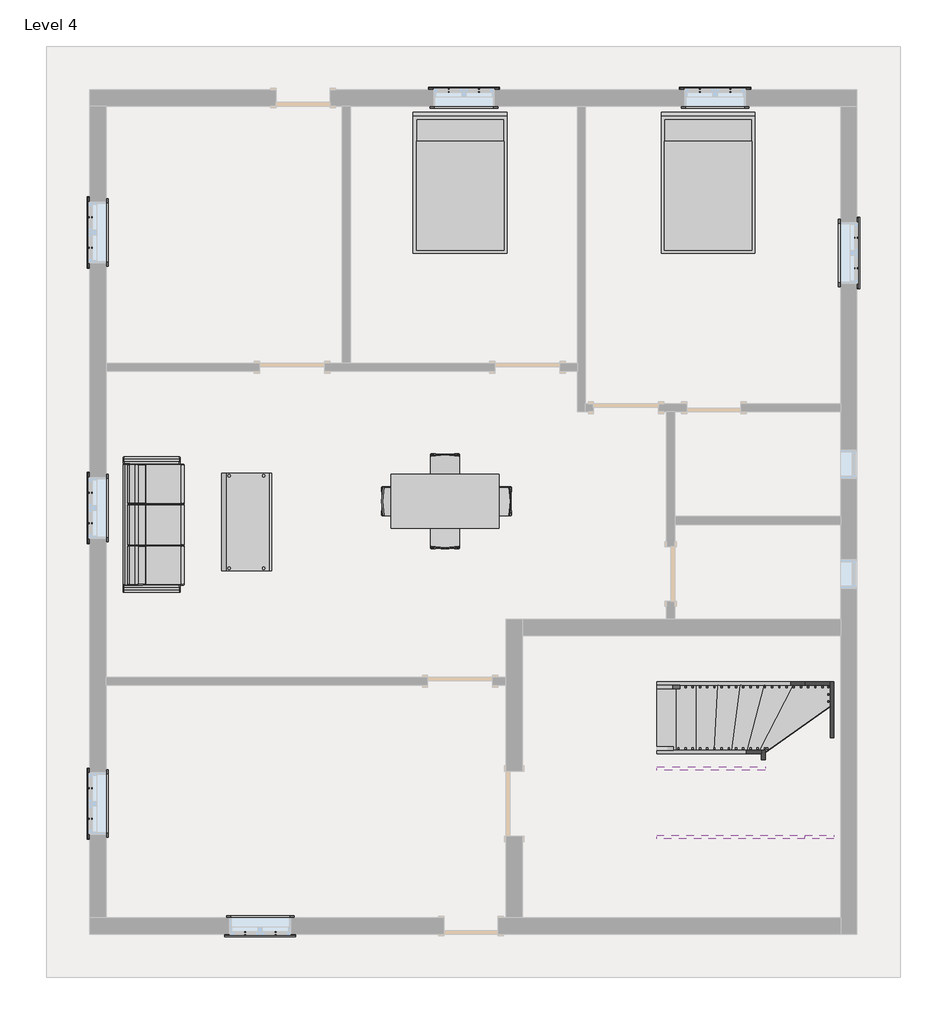
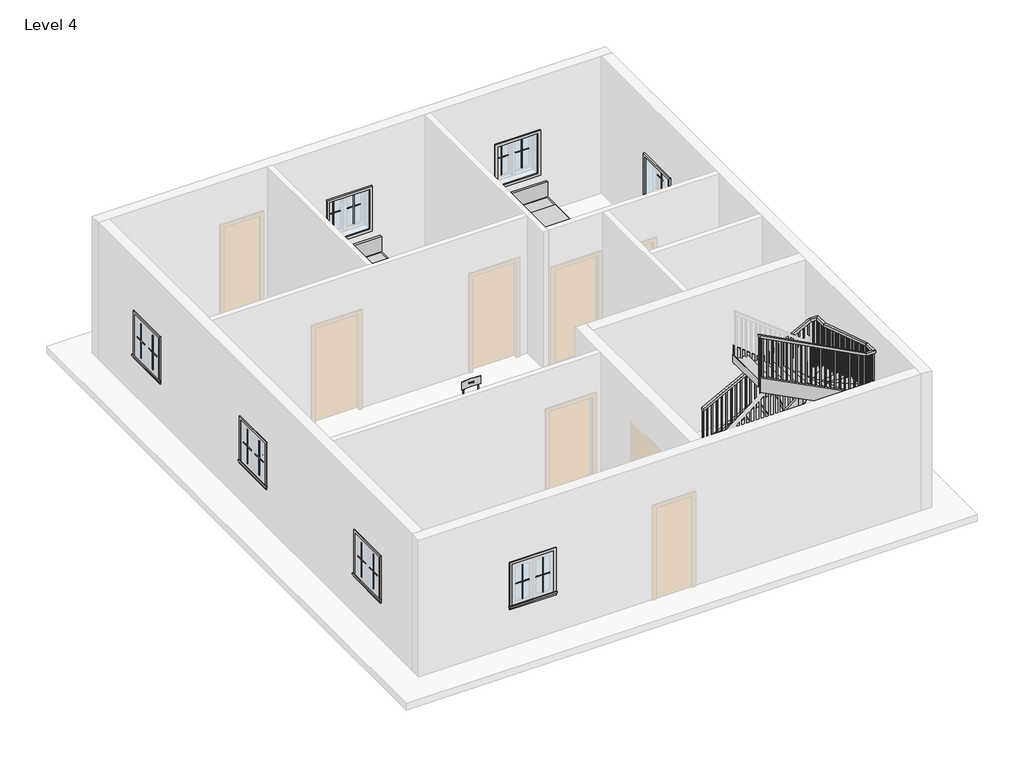
# One storey, part 2 of 2: 29 proxies, 8 members, 4 furniture elements, 1 railing, 1 stair flight.
"""IFC4 building model written with IfcOpenShell, lengths in millimetres."""

from ifc_helpers import new_model, si_unit, frame, origin, place, context, project, spatial, polyline, outline, extrude, faceted_brep, transform, mapped, element, save
from components import modern_coffee_table_17989_modern_coffee_table_17989_d3a860c8, muntin_pattern_2x2_muntin_pattern_2x2_b3fe6957, muntin_pattern_2x2_muntin_pattern_2x2_3e0ecaf2, trim_window_exterior_flat_with_sill_41619996, trim_window_interior_flat_picture_frame_51c85655, furniture_2fc85b74, furniture_29a9adb8, furniture_57072a26, bed_17739_bed_17739_15c61121, dining_table_w_chairs_11374_0cdfc61b, stair_flight_4d9189d9

model = new_model("IFC4")

# Units and contexts
model_context = context("Model", 3, world=origin())
ifc_project = project(units=[si_unit("LENGTHUNIT", "METRE", prefix="MILLI")], contexts=[model_context])

# Site, building, storey
site = spatial("IfcSite", under=ifc_project)
building = spatial("IfcBuilding", under=site)
storey = spatial("IfcBuildingStorey", under=building, Name="Level 4", Elevation=6400.8)

# Proxies
placement = place(None, origin())
modern_coffee_table_17989_modern_coffee_table_17989_shape = modern_coffee_table_17989_modern_coffee_table_17989_d3a860c8(model_context)
element("IfcBuildingElementProxy", 1, Name="Modern_Coffee_Table_17989 : Modern_Coffee_Table_17989", ObjectType="Modern_Coffee_Table_17989 : Modern_Coffee_Table_17989", at=placement, inside=storey, context=model_context, shape_type="MappedRepresentation", body=[
    mapped(modern_coffee_table_17989_modern_coffee_table_17989_shape, transform((-4791.7841049, 1283.3840961, 6400.8), x_axis=(0.0, 1.0, 0.0), y_axis=(-1.0, 0.0, 0.0), z_axis=(0.0, 0.0, 1.0))),
])
muntin_pattern_2x2_muntin_pattern_2x2_shape = muntin_pattern_2x2_muntin_pattern_2x2_b3fe6957(model_context)
element("IfcBuildingElementProxy", 2, Name="Muntin Pattern_2x2 : Muntin Pattern_2x2", ObjectType="Muntin Pattern_2x2 : Muntin Pattern_2x2", at=placement, inside=storey, context=model_context, shape_type="MappedRepresentation", body=[
    mapped(muntin_pattern_2x2_muntin_pattern_2x2_shape, transform((-1586.7442864, 7129.6784997, 7385.05), x_axis=(1.0, 0.0, 0.0), y_axis=(0.0, 1.0, 0.0), z_axis=(0.0, 0.0, 1.0))),
])
element("IfcBuildingElementProxy", 3, Name="Muntin Pattern_2x2 : Muntin Pattern_2x2", ObjectType="Muntin Pattern_2x2 : Muntin Pattern_2x2", at=placement, inside=storey, context=model_context, shape_type="MappedRepresentation", body=[
    mapped(muntin_pattern_2x2_muntin_pattern_2x2_shape, transform((1952.1107136, 7129.6784997, 7385.05), x_axis=(1.0, 0.0, 0.0), y_axis=(0.0, 1.0, 0.0), z_axis=(0.0, 0.0, 1.0))),
])
element("IfcBuildingElementProxy", 4, Name="Muntin Pattern_2x2 : Muntin Pattern_2x2", ObjectType="Muntin Pattern_2x2 : Muntin Pattern_2x2", at=placement, inside=storey, context=model_context, shape_type="MappedRepresentation", body=[
    mapped(muntin_pattern_2x2_muntin_pattern_2x2_shape, transform((-6633.4067864, 4915.1159997, 7385.05), x_axis=(0.0, 1.0, 0.0), y_axis=(-1.0, 0.0, 0.0), z_axis=(0.0, 0.0, 1.0))),
])
element("IfcBuildingElementProxy", 5, Name="Muntin Pattern_2x2 : Muntin Pattern_2x2", ObjectType="Muntin Pattern_2x2 : Muntin Pattern_2x2", at=placement, inside=storey, context=model_context, shape_type="MappedRepresentation", body=[
    mapped(muntin_pattern_2x2_muntin_pattern_2x2_shape, transform((-6633.4067864, 1038.4409997, 7385.05), x_axis=(0.0, 1.0, 0.0), y_axis=(-1.0, 0.0, 0.0), z_axis=(0.0, 0.0, 1.0))),
])
element("IfcBuildingElementProxy", 6, Name="Muntin Pattern_2x2 : Muntin Pattern_2x2", ObjectType="Muntin Pattern_2x2 : Muntin Pattern_2x2", at=placement, inside=storey, context=model_context, shape_type="MappedRepresentation", body=[
    mapped(muntin_pattern_2x2_muntin_pattern_2x2_shape, transform((4152.7032136, 5057.9909997, 7385.05), x_axis=(0.0, -1.0, 0.0), y_axis=(1.0, 0.0, 0.0), z_axis=(0.0, 0.0, 1.0))),
])
element("IfcBuildingElementProxy", 7, Name="Muntin Pattern_2x2 : Muntin Pattern_2x2", ObjectType="Muntin Pattern_2x2 : Muntin Pattern_2x2", at=placement, inside=storey, context=model_context, shape_type="MappedRepresentation", body=[
    mapped(muntin_pattern_2x2_muntin_pattern_2x2_shape, transform((-6633.4067864, -3125.2540003, 7385.05), x_axis=(0.0, 1.0, 0.0), y_axis=(-1.0, 0.0, 0.0), z_axis=(0.0, 0.0, 1.0))),
])
element("IfcBuildingElementProxy", 8, Name="Muntin Pattern_2x2 : Muntin Pattern_2x2", ObjectType="Muntin Pattern_2x2 : Muntin Pattern_2x2", at=placement, inside=storey, context=model_context, shape_type="MappedRepresentation", body=[
    mapped(muntin_pattern_2x2_muntin_pattern_2x2_shape, transform((-4028.3192864, -4738.4715003, 7385.05), x_axis=(-1.0, 0.0, 0.0), y_axis=(0.0, -1.0, 0.0), z_axis=(0.0, 0.0, 1.0))),
])
muntin_pattern_2x2_muntin_pattern_2x2_2_shape = muntin_pattern_2x2_muntin_pattern_2x2_3e0ecaf2(model_context)
element("IfcBuildingElementProxy", 9, Name="Muntin Pattern_2x2 : Muntin Pattern_2x2", ObjectType="Muntin Pattern_2x2 : Muntin Pattern_2x2", at=placement, inside=storey, context=model_context, shape_type="MappedRepresentation", body=[
    mapped(muntin_pattern_2x2_muntin_pattern_2x2_2_shape, transform((-1158.1192864, 7129.6784997, 7385.05), x_axis=(-1.0, 0.0, 0.0), y_axis=(0.0, -1.0, 0.0), z_axis=(0.0, 0.0, 1.0))),
])
element("IfcBuildingElementProxy", 10, Name="Muntin Pattern_2x2 : Muntin Pattern_2x2", ObjectType="Muntin Pattern_2x2 : Muntin Pattern_2x2", at=placement, inside=storey, context=model_context, shape_type="MappedRepresentation", body=[
    mapped(muntin_pattern_2x2_muntin_pattern_2x2_2_shape, transform((2380.7357136, 7129.6784997, 7385.05), x_axis=(-1.0, 0.0, 0.0), y_axis=(0.0, -1.0, 0.0), z_axis=(0.0, 0.0, 1.0))),
])
element("IfcBuildingElementProxy", 11, Name="Muntin Pattern_2x2 : Muntin Pattern_2x2", ObjectType="Muntin Pattern_2x2 : Muntin Pattern_2x2", at=placement, inside=storey, context=model_context, shape_type="MappedRepresentation", body=[
    mapped(muntin_pattern_2x2_muntin_pattern_2x2_2_shape, transform((-6633.4067864, 5343.7409997, 7385.05), x_axis=(0.0, -1.0, 0.0), y_axis=(1.0, 0.0, 0.0), z_axis=(0.0, 0.0, 1.0))),
])
element("IfcBuildingElementProxy", 12, Name="Muntin Pattern_2x2 : Muntin Pattern_2x2", ObjectType="Muntin Pattern_2x2 : Muntin Pattern_2x2", at=placement, inside=storey, context=model_context, shape_type="MappedRepresentation", body=[
    mapped(muntin_pattern_2x2_muntin_pattern_2x2_2_shape, transform((-6633.4067864, 1467.0659997, 7385.05), x_axis=(0.0, -1.0, 0.0), y_axis=(1.0, 0.0, 0.0), z_axis=(0.0, 0.0, 1.0))),
])
element("IfcBuildingElementProxy", 13, Name="Muntin Pattern_2x2 : Muntin Pattern_2x2", ObjectType="Muntin Pattern_2x2 : Muntin Pattern_2x2", at=placement, inside=storey, context=model_context, shape_type="MappedRepresentation", body=[
    mapped(muntin_pattern_2x2_muntin_pattern_2x2_2_shape, transform((4152.7032136, 4629.3659997, 7385.05), x_axis=(0.0, 1.0, 0.0), y_axis=(-1.0, 0.0, 0.0), z_axis=(0.0, 0.0, 1.0))),
])
element("IfcBuildingElementProxy", 14, Name="Muntin Pattern_2x2 : Muntin Pattern_2x2", ObjectType="Muntin Pattern_2x2 : Muntin Pattern_2x2", at=placement, inside=storey, context=model_context, shape_type="MappedRepresentation", body=[
    mapped(muntin_pattern_2x2_muntin_pattern_2x2_2_shape, transform((-6633.4067864, -2696.6290003, 7385.05), x_axis=(0.0, -1.0, 0.0), y_axis=(1.0, 0.0, 0.0), z_axis=(0.0, 0.0, 1.0))),
])
element("IfcBuildingElementProxy", 15, Name="Muntin Pattern_2x2 : Muntin Pattern_2x2", ObjectType="Muntin Pattern_2x2 : Muntin Pattern_2x2", at=placement, inside=storey, context=model_context, shape_type="MappedRepresentation", body=[
    mapped(muntin_pattern_2x2_muntin_pattern_2x2_2_shape, transform((-4456.9442864, -4738.4715003, 7385.05), x_axis=(1.0, 0.0, 0.0), y_axis=(0.0, 1.0, 0.0), z_axis=(0.0, 0.0, 1.0))),
])
trim_window_exterior_flat_with_sill_shape = trim_window_exterior_flat_with_sill_41619996(model_context)
element("IfcBuildingElementProxy", 16, Name="Trim-Window-Exterior-Flat : with Sill", ObjectType="Trim-Window-Exterior-Flat : with Sill", at=placement, inside=storey, context=model_context, shape_type="MappedRepresentation", body=[
    mapped(trim_window_exterior_flat_with_sill_shape, transform((-1372.4317864, 7139.2034997, 8229.6), x_axis=(-1.0, 0.0, 0.0), y_axis=(0.0, 0.0, 1.0), z_axis=(0.0, 1.0, 0.0))),
])
element("IfcBuildingElementProxy", 17, Name="Trim-Window-Exterior-Flat : with Sill", ObjectType="Trim-Window-Exterior-Flat : with Sill", at=placement, inside=storey, context=model_context, shape_type="MappedRepresentation", body=[
    mapped(trim_window_exterior_flat_with_sill_shape, transform((2166.4232136, 7139.2034997, 8229.6), x_axis=(-1.0, 0.0, 0.0), y_axis=(0.0, 0.0, 1.0), z_axis=(0.0, 1.0, 0.0))),
])
element("IfcBuildingElementProxy", 18, Name="Trim-Window-Exterior-Flat : with Sill", ObjectType="Trim-Window-Exterior-Flat : with Sill", at=placement, inside=storey, context=model_context, shape_type="MappedRepresentation", body=[
    mapped(trim_window_exterior_flat_with_sill_shape, transform((-6642.9317864, 5129.4284997, 8229.6), x_axis=(0.0, -1.0, 0.0), y_axis=(0.0, 0.0, 1.0), z_axis=(-1.0, 0.0, 0.0))),
])
element("IfcBuildingElementProxy", 19, Name="Trim-Window-Exterior-Flat : with Sill", ObjectType="Trim-Window-Exterior-Flat : with Sill", at=placement, inside=storey, context=model_context, shape_type="MappedRepresentation", body=[
    mapped(trim_window_exterior_flat_with_sill_shape, transform((-6642.9317864, 1252.7534997, 8229.6), x_axis=(0.0, -1.0, 0.0), y_axis=(0.0, 0.0, 1.0), z_axis=(-1.0, 0.0, 0.0))),
])
element("IfcBuildingElementProxy", 20, Name="Trim-Window-Exterior-Flat : with Sill", ObjectType="Trim-Window-Exterior-Flat : with Sill", at=placement, inside=storey, context=model_context, shape_type="MappedRepresentation", body=[
    mapped(trim_window_exterior_flat_with_sill_shape, transform((4162.2282136, 4843.6784997, 8229.6), x_axis=(0.0, 1.0, 0.0), y_axis=(0.0, 0.0, 1.0), z_axis=(1.0, 0.0, 0.0))),
])
element("IfcBuildingElementProxy", 21, Name="Trim-Window-Exterior-Flat : with Sill", ObjectType="Trim-Window-Exterior-Flat : with Sill", at=placement, inside=storey, context=model_context, shape_type="MappedRepresentation", body=[
    mapped(trim_window_exterior_flat_with_sill_shape, transform((-6642.9317864, -2910.9415003, 8229.6), x_axis=(0.0, -1.0, 0.0), y_axis=(0.0, 0.0, 1.0), z_axis=(-1.0, 0.0, 0.0))),
])
element("IfcBuildingElementProxy", 22, Name="Trim-Window-Exterior-Flat : with Sill", ObjectType="Trim-Window-Exterior-Flat : with Sill", at=placement, inside=storey, context=model_context, shape_type="MappedRepresentation", body=[
    mapped(trim_window_exterior_flat_with_sill_shape, transform((-4242.6317864, -4747.9965003, 8229.6), x_axis=(1.0, 0.0, 0.0), y_axis=(0.0, 0.0, 1.0), z_axis=(0.0, -1.0, 0.0))),
])
trim_window_interior_flat_picture_frame_shape = trim_window_interior_flat_picture_frame_51c85655(model_context)
element("IfcBuildingElementProxy", 23, Name="Trim-Window-Interior-Flat : Picture Frame", ObjectType="Trim-Window-Interior-Flat : Picture Frame", at=placement, inside=storey, context=model_context, shape_type="MappedRepresentation", body=[
    mapped(trim_window_interior_flat_picture_frame_shape, transform((-1372.4317864, 6910.6034997, 8229.6), x_axis=(1.0, 0.0, 0.0), y_axis=(0.0, 0.0, 1.0), z_axis=(0.0, -1.0, 0.0))),
])
element("IfcBuildingElementProxy", 24, Name="Trim-Window-Interior-Flat : Picture Frame", ObjectType="Trim-Window-Interior-Flat : Picture Frame", at=placement, inside=storey, context=model_context, shape_type="MappedRepresentation", body=[
    mapped(trim_window_interior_flat_picture_frame_shape, transform((2166.4232136, 6910.6034997, 8229.6), x_axis=(1.0, 0.0, 0.0), y_axis=(0.0, 0.0, 1.0), z_axis=(0.0, -1.0, 0.0))),
])
element("IfcBuildingElementProxy", 25, Name="Trim-Window-Interior-Flat : Picture Frame", ObjectType="Trim-Window-Interior-Flat : Picture Frame", at=placement, inside=storey, context=model_context, shape_type="MappedRepresentation", body=[
    mapped(trim_window_interior_flat_picture_frame_shape, transform((-6414.3317864, 5129.4284997, 8229.6), x_axis=(0.0, 1.0, 0.0), y_axis=(0.0, 0.0, 1.0), z_axis=(1.0, 0.0, 0.0))),
])
element("IfcBuildingElementProxy", 26, Name="Trim-Window-Interior-Flat : Picture Frame", ObjectType="Trim-Window-Interior-Flat : Picture Frame", at=placement, inside=storey, context=model_context, shape_type="MappedRepresentation", body=[
    mapped(trim_window_interior_flat_picture_frame_shape, transform((-6414.3317864, 1252.7534997, 8229.6), x_axis=(0.0, 1.0, 0.0), y_axis=(0.0, 0.0, 1.0), z_axis=(1.0, 0.0, 0.0))),
])
element("IfcBuildingElementProxy", 27, Name="Trim-Window-Interior-Flat : Picture Frame", ObjectType="Trim-Window-Interior-Flat : Picture Frame", at=placement, inside=storey, context=model_context, shape_type="MappedRepresentation", body=[
    mapped(trim_window_interior_flat_picture_frame_shape, transform((3933.6282136, 4843.6784997, 8229.6), x_axis=(0.0, -1.0, 0.0), y_axis=(0.0, 0.0, 1.0), z_axis=(-1.0, 0.0, 0.0))),
])
element("IfcBuildingElementProxy", 28, Name="Trim-Window-Interior-Flat : Picture Frame", ObjectType="Trim-Window-Interior-Flat : Picture Frame", at=placement, inside=storey, context=model_context, shape_type="MappedRepresentation", body=[
    mapped(trim_window_interior_flat_picture_frame_shape, transform((-6414.3317864, -2910.9415003, 8229.6), x_axis=(0.0, 1.0, 0.0), y_axis=(0.0, 0.0, 1.0), z_axis=(1.0, 0.0, 0.0))),
])
element("IfcBuildingElementProxy", 29, Name="Trim-Window-Interior-Flat : Picture Frame", ObjectType="Trim-Window-Interior-Flat : Picture Frame", at=placement, inside=storey, context=model_context, shape_type="MappedRepresentation", body=[
    mapped(trim_window_interior_flat_picture_frame_shape, transform((-4242.6317864, -4519.3965003, 8229.6), x_axis=(-1.0, 0.0, 0.0), y_axis=(0.0, 0.0, 1.0), z_axis=(0.0, 1.0, 0.0))),
])

# Furniture
furniture_shape = furniture_2fc85b74(model_context)
furniture_2_shape = furniture_29a9adb8(model_context)
furniture_3_shape = furniture_57072a26(model_context)
element("IfcFurniture", 30, at=placement, inside=storey, context=model_context, shape_type="MappedRepresentation", body=[
    mapped(furniture_shape, transform((-5371.0104604, 1017.8034997, 6400.8), x_axis=(0.0, 1.0, 0.0), y_axis=(-1.0, 0.0, 0.0), z_axis=(0.0, 0.0, 1.0))),
    mapped(furniture_2_shape, transform((-5371.0104604, 1017.8034997, 6400.8), x_axis=(0.0, 1.0, 0.0), y_axis=(-1.0, 0.0, 0.0), z_axis=(0.0, 0.0, 1.0))),
    mapped(furniture_3_shape, transform((-5371.0104604, 1017.8034997, 6400.8), x_axis=(0.0, 1.0, 0.0), y_axis=(-1.0, 0.0, 0.0), z_axis=(0.0, 0.0, 1.0))),
])
bed_17739_bed_17739_shape = bed_17739_bed_17739_15c61121(model_context)
element("IfcFurniture", 31, ObjectType="Bed_17739 : Bed_17739", at=placement, inside=storey, context=model_context, shape_type="MappedRepresentation", body=[
    mapped(bed_17739_bed_17739_shape, transform((-1425.7717864, 5805.7034997, 6400.8), x_axis=(1.0, 0.0, 0.0), y_axis=(0.0, 1.0, 0.0), z_axis=(0.0, 0.0, 1.0))),
])
element("IfcFurniture", 32, ObjectType="Bed_17739 : Bed_17739", at=placement, inside=storey, context=model_context, shape_type="MappedRepresentation", body=[
    mapped(bed_17739_bed_17739_shape, transform((2066.7282136, 5805.7034997, 6400.8), x_axis=(1.0, 0.0, 0.0), y_axis=(0.0, 1.0, 0.0), z_axis=(0.0, 0.0, 1.0))),
])
dining_table_w_chairs_11374_shape = dining_table_w_chairs_11374_0cdfc61b(model_context)
element("IfcFurniture", 33, ObjectType="Dining_Table_w_Chairs_11374", at=placement, inside=storey, context=model_context, shape_type="MappedRepresentation", body=[
    mapped(dining_table_w_chairs_11374_shape, transform((-1657.0397106, 1252.0888157, 6400.8), x_axis=(1.0, 0.0, 0.0), y_axis=(0.0, 1.0, 0.0), z_axis=(0.0, 0.0, 1.0))),
])

# Members
element("IfcMember", 34, ObjectType="Stringer - 2\" Width", at=placement, inside=storey, context=model_context, shape_type="SweptSolid", body=[
    extrude(outline(polyline([(6630.439954, 1342.8282136), (6400.8, 1342.8282136), (6400.8, 1562.5905312), (7363.300629, 3430.2454053), (7706.1956453, 3430.2454053), (6630.439954, 1342.8282136)])), frame((0.0, -1245.3365003, 0.0), z_axis=(0.0, 1.0, 0.0), x_axis=(0.0, 0.0, 1.0)), (0.0, 0.0, 1.0), 50.8),
])
element("IfcMember", 35, ObjectType="Stringer - 2\" Width", at=placement, inside=storey, context=model_context, shape_type="SweptSolid", body=[
    extrude(outline(polyline([(3430.2454053, -1245.3365003), (3430.2454053, -1194.5365003), (3784.9599055, -1194.5365003), (3784.9599055, -1245.3365003), (3430.2454053, -1245.3365003)])), frame((0.0, 0.0, 7363.300629), z_axis=(0.0, 0.0, 1.0), x_axis=(1.0, 0.0, 0.0)), (0.0, 0.0, 1.0), 342.8950162),
])
element("IfcMember", 36, ObjectType="Stringer - 2\" Width", at=placement, inside=storey, context=model_context, shape_type="SweptSolid", body=[
    extrude(outline(polyline([(-1194.5365003, 7689.8952212), (-1194.5365003, 7401.3956453), (-1364.0589833, 7401.3956453), (-3353.5365003, 8039.7682298), (-3353.5365003, 8370.7972697), (-3316.5563831, 8370.7972697), (-1194.5365003, 7689.8952212)])), frame((3784.9599055, 0.0, 0.0), z_axis=(1.0, 0.0, 0.0), x_axis=(0.0, 1.0, 0.0)), (0.0, 0.0, 1.0), 50.8),
])
element("IfcMember", 37, ObjectType="Stringer - 2\" Width", at=placement, inside=storey, context=model_context, shape_type="SweptSolid", body=[
    extrude(outline(polyline([(3835.7599055, -3353.5365003), (3835.7599055, -3404.3365003), (3430.2454053, -3404.3365003), (3430.2454053, -3353.5365003), (3835.7599055, -3353.5365003)])), frame((0.0, 0.0, 8050.6904473), z_axis=(0.0, 0.0, 1.0), x_axis=(1.0, 0.0, 0.0)), (0.0, 0.0, 1.0), 320.1068224),
])
element("IfcMember", 38, ObjectType="Stringer - 2\" Width", at=placement, inside=storey, context=model_context, shape_type="SweptSolid", body=[
    extrude(outline(polyline([(8050.6904473, 3430.2454053), (8370.7972697, 3430.2454053), (9446.5529609, 1342.8282136), (9126.4461385, 1342.8282136), (8050.6904473, 3430.2454053)])), frame((0.0, -3404.3365003, 0.0), z_axis=(0.0, 1.0, 0.0), x_axis=(0.0, 0.0, 1.0)), (0.0, 0.0, 1.0), 50.8),
])
element("IfcMember", 39, ObjectType="Stringer - 2\" Width", at=placement, inside=storey, context=model_context, shape_type="SweptSolid", body=[
    extrude(outline(polyline([(6576.9764461, 1342.8282136), (6400.8, 1342.8282136), (6400.8, 1609.0898582), (7387.9410923, 2819.7599055), (7781.218648, 2819.7599055), (6576.9764461, 1342.8282136)])), frame((0.0, -2210.5365003, 0.0), z_axis=(0.0, 1.0, 0.0), x_axis=(0.0, 0.0, 1.0)), (0.0, 0.0, 1.0), 50.8),
])
element("IfcMember", 40, ObjectType="Stringer - 2\" Width", at=placement, inside=storey, context=model_context, shape_type="SweptSolid", body=[
    extrude(outline(polyline([(-2159.7365003, 7974.0682978), (-2159.7365003, 7429.3617647), (-2193.9787177, 7429.3617647), (-2388.3365003, 7761.265107), (-2388.3365003, 8326.9409689), (-2366.3736178, 8326.9409689), (-2159.7365003, 7974.0682978)])), frame((2819.7599055, 0.0, 0.0), z_axis=(1.0, 0.0, 0.0), x_axis=(0.0, 1.0, 0.0)), (0.0, 0.0, 1.0), 50.8),
])
element("IfcMember", 41, ObjectType="Stringer - 2\" Width", at=placement, inside=storey, context=model_context, shape_type="SweptSolid", body=[
    extrude(outline(polyline([(7933.6634131, 2870.5599055), (8326.9409689, 2870.5599055), (9572.6038432, 1342.8282136), (9179.3262875, 1342.8282136), (7933.6634131, 2870.5599055)])), frame((0.0, -2439.1365003, 0.0), z_axis=(0.0, 1.0, 0.0), x_axis=(0.0, 0.0, 1.0)), (0.0, 0.0, 1.0), 50.8),
])

# Railing
element("IfcRailing", 42, ObjectType="Handrail - Rectangular", at=placement, inside=storey, context=model_context, shape_type="SolidModel", body=[
    faceted_brep([(1342.8282136, -1245.3365003, 7484.5333333), (1342.8282136, -1245.3365003, 7427.0742652), (1342.8282136, -1296.1365003, 7427.0742652), (1342.8282136, -1296.1365003, 7484.5333333), (3600.5532757, -1245.3365003, 8677.8239201), (3613.1523402, -1245.3365003, 8627.0239201), (3613.1523402, -1296.1365003, 8627.0239201), (3600.5532757, -1296.1365003, 8677.8239201), (3784.9599055, -1245.3365003, 8677.8239201), (3784.9599055, -1245.3365003, 8627.0239201), (3734.1599055, -1296.1365003, 8627.0239201), (3734.1599055, -1296.1365003, 8677.8239201), (3784.9599055, -1532.6483825, 8677.8239201), (3784.9599055, -1540.5989586, 8627.0239201), (3734.1599055, -1540.5989586, 8627.0239201), (3734.1599055, -1532.6483825, 8677.8239201), (3784.9599055, -3066.2246182, 9169.9094132), (3784.9599055, -3074.1751943, 9119.1094132), (3734.1599055, -3074.1751943, 9119.1094132), (3734.1599055, -3066.2246182, 9169.9094132), (3784.9599055, -3353.5365003, 9169.9094132), (3784.9599055, -3353.5365003, 9119.1094132), (3734.1599055, -3302.7365003, 9119.1094132), (3734.1599055, -3302.7365003, 9169.9094132), (3600.5532757, -3353.5365003, 9169.9094132), (3587.9542112, -3353.5365003, 9119.1094132), (3587.9542112, -3302.7365003, 9119.1094132), (3600.5532757, -3302.7365003, 9169.9094132), (1342.8282136, -3353.5365003, 10363.2), (1342.8282136, -3302.7365003, 10363.2), (1342.8282136, -3302.7365003, 10305.7409318), (1342.8282136, -3353.5365003, 10305.7409318)], [[[0, 1, 2, 3]], [[1, 0, 4, 5]], [[2, 1, 5, 6]], [[3, 2, 6, 7]], [[0, 3, 7, 4]], [[5, 4, 8, 9]], [[6, 5, 9, 10]], [[7, 6, 10, 11]], [[4, 7, 11, 8]], [[9, 8, 12, 13]], [[10, 9, 13, 14]], [[11, 10, 14, 15]], [[8, 11, 15, 12]], [[13, 12, 16, 17]], [[14, 13, 17, 18]], [[15, 14, 18, 19]], [[12, 15, 19, 16]], [[17, 16, 20, 21]], [[18, 17, 21, 22]], [[19, 18, 22, 23]], [[16, 19, 23, 20]], [[21, 20, 24, 25]], [[22, 21, 25, 26]], [[23, 22, 26, 27]], [[20, 23, 27, 24]], [[28, 29, 30, 31]], [[25, 24, 28, 31]], [[26, 25, 31, 30]], [[27, 26, 30, 29]], [[24, 27, 29, 28]]]),
    extrude(outline(polyline([(10268.5284102, 1413.2349055), (9279.4666667, 1413.2349055), (9279.4666667, 1432.2849055), (10258.4597858, 1432.2849055), (10268.5284102, 1413.2349055)])), frame((0.0, -3337.6615003, 0.0), z_axis=(0.0, 1.0, 0.0), x_axis=(0.0, 0.0, 1.0)), (0.0, 0.0, 1.0), 19.05),
    extrude(outline(polyline([(10214.82908, 1514.8349055), (9279.4666667, 1514.8349055), (9279.4666667, 1533.8849055), (10204.7604556, 1533.8849055), (10214.82908, 1514.8349055)])), frame((0.0, -3337.6615003, 0.0), z_axis=(0.0, 1.0, 0.0), x_axis=(0.0, 0.0, 1.0)), (0.0, 0.0, 1.0), 19.05),
    extrude(outline(polyline([(10161.1297498, 1616.4349055), (9110.1333333, 1616.4349055), (9110.1333333, 1635.4849055), (10151.0611254, 1635.4849055), (10161.1297498, 1616.4349055)])), frame((0.0, -3337.6615003, 0.0), z_axis=(0.0, 1.0, 0.0), x_axis=(0.0, 0.0, 1.0)), (0.0, 0.0, 1.0), 19.05),
    extrude(outline(polyline([(10107.4304196, 1718.0349055), (9110.1333333, 1718.0349055), (9110.1333333, 1737.0849055), (10097.3617952, 1737.0849055), (10107.4304196, 1718.0349055)])), frame((0.0, -3337.6615003, 0.0), z_axis=(0.0, 1.0, 0.0), x_axis=(0.0, 0.0, 1.0)), (0.0, 0.0, 1.0), 19.05),
    extrude(outline(polyline([(10053.7310894, 1819.6349055), (9110.1333333, 1819.6349055), (9110.1333333, 1838.6849055), (10043.662465, 1838.6849055), (10053.7310894, 1819.6349055)])), frame((0.0, -3337.6615003, 0.0), z_axis=(0.0, 1.0, 0.0), x_axis=(0.0, 0.0, 1.0)), (0.0, 0.0, 1.0), 19.05),
    extrude(outline(polyline([(10000.0317592, 1921.2349055), (8940.8, 1921.2349055), (8940.8, 1940.2849055), (9989.9631348, 1940.2849055), (10000.0317592, 1921.2349055)])), frame((0.0, -3337.6615003, 0.0), z_axis=(0.0, 1.0, 0.0), x_axis=(0.0, 0.0, 1.0)), (0.0, 0.0, 1.0), 19.05),
    extrude(outline(polyline([(9946.332429, 2022.8349055), (8940.8, 2022.8349055), (8940.8, 2041.8849055), (9936.2638046, 2041.8849055), (9946.332429, 2022.8349055)])), frame((0.0, -3337.6615003, 0.0), z_axis=(0.0, 1.0, 0.0), x_axis=(0.0, 0.0, 1.0)), (0.0, 0.0, 1.0), 19.05),
    extrude(outline(polyline([(9892.6330988, 2124.4349055), (8940.8, 2124.4349055), (8940.8, 2143.4849055), (9882.5644744, 2143.4849055), (9892.6330988, 2124.4349055)])), frame((0.0, -3337.6615003, 0.0), z_axis=(0.0, 1.0, 0.0), x_axis=(0.0, 0.0, 1.0)), (0.0, 0.0, 1.0), 19.05),
    extrude(outline(polyline([(9838.9337686, 2226.0349055), (8771.4666667, 2226.0349055), (8771.4666667, 2245.0849055), (9828.8651442, 2245.0849055), (9838.9337686, 2226.0349055)])), frame((0.0, -3337.6615003, 0.0), z_axis=(0.0, 1.0, 0.0), x_axis=(0.0, 0.0, 1.0)), (0.0, 0.0, 1.0), 19.05),
    extrude(outline(polyline([(9785.2344384, 2327.6349055), (8771.4666667, 2327.6349055), (8771.4666667, 2346.6849055), (9775.165814, 2346.6849055), (9785.2344384, 2327.6349055)])), frame((0.0, -3337.6615003, 0.0), z_axis=(0.0, 1.0, 0.0), x_axis=(0.0, 0.0, 1.0)), (0.0, 0.0, 1.0), 19.05),
    extrude(outline(polyline([(9731.5351082, 2429.2349055), (8771.4666667, 2429.2349055), (8771.4666667, 2448.2849055), (9721.4664838, 2448.2849055), (9731.5351082, 2429.2349055)])), frame((0.0, -3337.6615003, 0.0), z_axis=(0.0, 1.0, 0.0), x_axis=(0.0, 0.0, 1.0)), (0.0, 0.0, 1.0), 19.05),
    extrude(outline(polyline([(9677.835778, 2530.8349055), (8602.1333333, 2530.8349055), (8602.1333333, 2549.8849055), (9667.7671536, 2549.8849055), (9677.835778, 2530.8349055)])), frame((0.0, -3337.6615003, 0.0), z_axis=(0.0, 1.0, 0.0), x_axis=(0.0, 0.0, 1.0)), (0.0, 0.0, 1.0), 19.05),
    extrude(outline(polyline([(9624.1364478, 2632.4349055), (8602.1333333, 2632.4349055), (8602.1333333, 2651.4849055), (9614.0678234, 2651.4849055), (9624.1364478, 2632.4349055)])), frame((0.0, -3337.6615003, 0.0), z_axis=(0.0, 1.0, 0.0), x_axis=(0.0, 0.0, 1.0)), (0.0, 0.0, 1.0), 19.05),
    extrude(outline(polyline([(9570.4371176, 2734.0349055), (8602.1333333, 2734.0349055), (8602.1333333, 2753.0849055), (9560.3684932, 2753.0849055), (9570.4371176, 2734.0349055)])), frame((0.0, -3337.6615003, 0.0), z_axis=(0.0, 1.0, 0.0), x_axis=(0.0, 0.0, 1.0)), (0.0, 0.0, 1.0), 19.05),
    extrude(outline(polyline([(9516.7377874, 2835.6349055), (8602.1333333, 2835.6349055), (8602.1333333, 2854.6849055), (9506.669163, 2854.6849055), (9516.7377874, 2835.6349055)])), frame((0.0, -3337.6615003, 0.0), z_axis=(0.0, 1.0, 0.0), x_axis=(0.0, 0.0, 1.0)), (0.0, 0.0, 1.0), 19.05),
    extrude(outline(polyline([(9463.0384572, 2937.2349055), (8432.8, 2937.2349055), (8432.8, 2956.2849055), (9452.9698328, 2956.2849055), (9463.0384572, 2937.2349055)])), frame((0.0, -3337.6615003, 0.0), z_axis=(0.0, 1.0, 0.0), x_axis=(0.0, 0.0, 1.0)), (0.0, 0.0, 1.0), 19.05),
    extrude(outline(polyline([(9409.339127, 3038.8349055), (8432.8, 3038.8349055), (8432.8, 3057.8849055), (9399.2705026, 3057.8849055), (9409.339127, 3038.8349055)])), frame((0.0, -3337.6615003, 0.0), z_axis=(0.0, 1.0, 0.0), x_axis=(0.0, 0.0, 1.0)), (0.0, 0.0, 1.0), 19.05),
    extrude(outline(polyline([(9355.6397968, 3140.4349055), (8432.8, 3140.4349055), (8432.8, 3159.4849055), (9345.5711724, 3159.4849055), (9355.6397968, 3140.4349055)])), frame((0.0, -3337.6615003, 0.0), z_axis=(0.0, 1.0, 0.0), x_axis=(0.0, 0.0, 1.0)), (0.0, 0.0, 1.0), 19.05),
    extrude(outline(polyline([(9301.9404666, 3242.0349055), (8432.8, 3242.0349055), (8432.8, 3261.0849055), (9291.8718422, 3261.0849055), (9301.9404666, 3242.0349055)])), frame((0.0, -3337.6615003, 0.0), z_axis=(0.0, 1.0, 0.0), x_axis=(0.0, 0.0, 1.0)), (0.0, 0.0, 1.0), 19.05),
    extrude(outline(polyline([(9248.2411364, 3343.6349055), (8263.4666667, 3343.6349055), (8263.4666667, 3362.6849055), (9238.172512, 3362.6849055), (9248.2411364, 3343.6349055)])), frame((0.0, -3337.6615003, 0.0), z_axis=(0.0, 1.0, 0.0), x_axis=(0.0, 0.0, 1.0)), (0.0, 0.0, 1.0), 19.05),
    extrude(outline(polyline([(9194.5418062, 3445.2349055), (8263.4666667, 3445.2349055), (8263.4666667, 3464.2849055), (9184.4731818, 3464.2849055), (9194.5418062, 3445.2349055)])), frame((0.0, -3337.6615003, 0.0), z_axis=(0.0, 1.0, 0.0), x_axis=(0.0, 0.0, 1.0)), (0.0, 0.0, 1.0), 19.05),
    extrude(outline(polyline([(9140.842476, 3546.8349055), (8263.4666667, 3546.8349055), (8263.4666667, 3565.8849055), (9130.7738516, 3565.8849055), (9140.842476, 3546.8349055)])), frame((0.0, -3337.6615003, 0.0), z_axis=(0.0, 1.0, 0.0), x_axis=(0.0, 0.0, 1.0)), (0.0, 0.0, 1.0), 19.05),
    extrude(outline(polyline([(3667.4849055, -3337.6615003), (3648.4349055, -3337.6615003), (3648.4349055, -3318.6115003), (3667.4849055, -3318.6115003), (3667.4849055, -3337.6615003)])), frame((0.0, 0.0, 8263.4666667), z_axis=(0.0, 0.0, 1.0), x_axis=(1.0, 0.0, 0.0)), (0.0, 0.0, 1.0), 855.6427466),
    extrude(outline(polyline([(3769.0849055, -3293.2115003), (3769.0849055, -3312.2615003), (3750.0349055, -3312.2615003), (3750.0349055, -3293.2115003), (3769.0849055, -3293.2115003)])), frame((0.0, 0.0, 8263.4666667), z_axis=(0.0, 0.0, 1.0), x_axis=(1.0, 0.0, 0.0)), (0.0, 0.0, 1.0), 855.6427466),
    extrude(outline(polyline([(3769.0849055, -3191.6115003), (3769.0849055, -3210.6615003), (3750.0349055, -3210.6615003), (3750.0349055, -3191.6115003), (3769.0849055, -3191.6115003)])), frame((0.0, 0.0, 8263.4666667), z_axis=(0.0, 0.0, 1.0), x_axis=(1.0, 0.0, 0.0)), (0.0, 0.0, 1.0), 855.6427466),
    extrude(outline(polyline([(3769.0849055, -3090.0115003), (3769.0849055, -3109.0615003), (3750.0349055, -3109.0615003), (3750.0349055, -3090.0115003), (3769.0849055, -3090.0115003)])), frame((0.0, 0.0, 8263.4666667), z_axis=(0.0, 0.0, 1.0), x_axis=(1.0, 0.0, 0.0)), (0.0, 0.0, 1.0), 855.6427466),
    extrude(outline(polyline([(-2988.4115003, 9091.5900316), (-2988.4115003, 8094.1333333), (-3007.4615003, 8094.1333333), (-3007.4615003, 9097.7026907), (-2988.4115003, 9091.5900316)])), frame((3750.0349055, 0.0, 0.0), z_axis=(1.0, 0.0, 0.0), x_axis=(0.0, 1.0, 0.0)), (0.0, 0.0, 1.0), 19.05),
    extrude(outline(polyline([(-2886.8115003, 9058.9891834), (-2886.8115003, 8094.1333333), (-2905.8615003, 8094.1333333), (-2905.8615003, 9065.1018425), (-2886.8115003, 9058.9891834)])), frame((3750.0349055, 0.0, 0.0), z_axis=(1.0, 0.0, 0.0), x_axis=(0.0, 1.0, 0.0)), (0.0, 0.0, 1.0), 19.05),
    extrude(outline(polyline([(-2785.2115003, 9026.3883352), (-2785.2115003, 8094.1333333), (-2804.2615003, 8094.1333333), (-2804.2615003, 9032.5009942), (-2785.2115003, 9026.3883352)])), frame((3750.0349055, 0.0, 0.0), z_axis=(1.0, 0.0, 0.0), x_axis=(0.0, 1.0, 0.0)), (0.0, 0.0, 1.0), 19.05),
    extrude(outline(polyline([(-2683.6115003, 8993.787487), (-2683.6115003, 8094.1333333), (-2702.6615003, 8094.1333333), (-2702.6615003, 8999.900146), (-2683.6115003, 8993.787487)])), frame((3750.0349055, 0.0, 0.0), z_axis=(1.0, 0.0, 0.0), x_axis=(0.0, 1.0, 0.0)), (0.0, 0.0, 1.0), 19.05),
    extrude(outline(polyline([(-2582.0115003, 8961.1866387), (-2582.0115003, 8094.1333333), (-2601.0615003, 8094.1333333), (-2601.0615003, 8967.2992978), (-2582.0115003, 8961.1866387)])), frame((3750.0349055, 0.0, 0.0), z_axis=(1.0, 0.0, 0.0), x_axis=(0.0, 1.0, 0.0)), (0.0, 0.0, 1.0), 19.05),
    extrude(outline(polyline([(-2480.4115003, 8928.5857905), (-2480.4115003, 7924.8), (-2499.4615003, 7924.8), (-2499.4615003, 8934.6984495), (-2480.4115003, 8928.5857905)])), frame((3750.0349055, 0.0, 0.0), z_axis=(1.0, 0.0, 0.0), x_axis=(0.0, 1.0, 0.0)), (0.0, 0.0, 1.0), 19.05),
    extrude(outline(polyline([(-2378.8115003, 8895.9849423), (-2378.8115003, 7924.8), (-2397.8615003, 7924.8), (-2397.8615003, 8902.0976013), (-2378.8115003, 8895.9849423)])), frame((3750.0349055, 0.0, 0.0), z_axis=(1.0, 0.0, 0.0), x_axis=(0.0, 1.0, 0.0)), (0.0, 0.0, 1.0), 19.05),
    extrude(outline(polyline([(-2277.2115003, 8863.384094), (-2277.2115003, 7924.8), (-2296.2615003, 7924.8), (-2296.2615003, 8869.4967531), (-2277.2115003, 8863.384094)])), frame((3750.0349055, 0.0, 0.0), z_axis=(1.0, 0.0, 0.0), x_axis=(0.0, 1.0, 0.0)), (0.0, 0.0, 1.0), 19.05),
    extrude(outline(polyline([(-2175.6115003, 8830.7832458), (-2175.6115003, 7924.8), (-2194.6615003, 7924.8), (-2194.6615003, 8836.8959049), (-2175.6115003, 8830.7832458)])), frame((3750.0349055, 0.0, 0.0), z_axis=(1.0, 0.0, 0.0), x_axis=(0.0, 1.0, 0.0)), (0.0, 0.0, 1.0), 19.05),
    extrude(outline(polyline([(-2074.0115003, 8798.1823976), (-2074.0115003, 7924.8), (-2093.0615003, 7924.8), (-2093.0615003, 8804.2950566), (-2074.0115003, 8798.1823976)])), frame((3750.0349055, 0.0, 0.0), z_axis=(1.0, 0.0, 0.0), x_axis=(0.0, 1.0, 0.0)), (0.0, 0.0, 1.0), 19.05),
    extrude(outline(polyline([(-1972.4115003, 8765.5815494), (-1972.4115003, 7755.4666667), (-1991.4615003, 7755.4666667), (-1991.4615003, 8771.6942084), (-1972.4115003, 8765.5815494)])), frame((3750.0349055, 0.0, 0.0), z_axis=(1.0, 0.0, 0.0), x_axis=(0.0, 1.0, 0.0)), (0.0, 0.0, 1.0), 19.05),
    extrude(outline(polyline([(-1870.8115003, 8732.9807011), (-1870.8115003, 7755.4666667), (-1889.8615003, 7755.4666667), (-1889.8615003, 8739.0933602), (-1870.8115003, 8732.9807011)])), frame((3750.0349055, 0.0, 0.0), z_axis=(1.0, 0.0, 0.0), x_axis=(0.0, 1.0, 0.0)), (0.0, 0.0, 1.0), 19.05),
    extrude(outline(polyline([(-1769.2115003, 8700.3798529), (-1769.2115003, 7755.4666667), (-1788.2615003, 7755.4666667), (-1788.2615003, 8706.492512), (-1769.2115003, 8700.3798529)])), frame((3750.0349055, 0.0, 0.0), z_axis=(1.0, 0.0, 0.0), x_axis=(0.0, 1.0, 0.0)), (0.0, 0.0, 1.0), 19.05),
    extrude(outline(polyline([(-1667.6115003, 8667.7790047), (-1667.6115003, 7755.4666667), (-1686.6615003, 7755.4666667), (-1686.6615003, 8673.8916637), (-1667.6115003, 8667.7790047)])), frame((3750.0349055, 0.0, 0.0), z_axis=(1.0, 0.0, 0.0), x_axis=(0.0, 1.0, 0.0)), (0.0, 0.0, 1.0), 19.05),
    extrude(outline(polyline([(-1566.0115003, 8635.1781565), (-1566.0115003, 7755.4666667), (-1585.0615003, 7755.4666667), (-1585.0615003, 8641.2908155), (-1566.0115003, 8635.1781565)])), frame((3750.0349055, 0.0, 0.0), z_axis=(1.0, 0.0, 0.0), x_axis=(0.0, 1.0, 0.0)), (0.0, 0.0, 1.0), 19.05),
    extrude(outline(polyline([(3769.0849055, -1464.4115003), (3769.0849055, -1483.4615003), (3750.0349055, -1483.4615003), (3750.0349055, -1464.4115003), (3769.0849055, -1464.4115003)])), frame((0.0, 0.0, 7586.1333333), z_axis=(0.0, 0.0, 1.0), x_axis=(1.0, 0.0, 0.0)), (0.0, 0.0, 1.0), 1040.8905868),
    extrude(outline(polyline([(3769.0849055, -1362.8115003), (3769.0849055, -1381.8615003), (3750.0349055, -1381.8615003), (3750.0349055, -1362.8115003), (3769.0849055, -1362.8115003)])), frame((0.0, 0.0, 7586.1333333), z_axis=(0.0, 0.0, 1.0), x_axis=(1.0, 0.0, 0.0)), (0.0, 0.0, 1.0), 1040.8905868),
    extrude(outline(polyline([(3670.1032136, -1261.2115003), (3689.1532136, -1261.2115003), (3689.1532136, -1280.2615003), (3670.1032136, -1280.2615003), (3670.1032136, -1261.2115003)])), frame((0.0, 0.0, 7586.1333333), z_axis=(0.0, 0.0, 1.0), x_axis=(1.0, 0.0, 0.0)), (0.0, 0.0, 1.0), 1040.8905868),
    extrude(outline(polyline([(8603.4252174, 3568.5032136), (7586.1333333, 3568.5032136), (7586.1333333, 3587.5532136), (8613.4938418, 3587.5532136), (8603.4252174, 3568.5032136)])), frame((0.0, -1280.2615003, 0.0), z_axis=(0.0, 1.0, 0.0), x_axis=(0.0, 0.0, 1.0)), (0.0, 0.0, 1.0), 19.05),
    extrude(outline(polyline([(8549.7258872, 3466.9032136), (7586.1333333, 3466.9032136), (7586.1333333, 3485.9532136), (8559.7945116, 3485.9532136), (8549.7258872, 3466.9032136)])), frame((0.0, -1280.2615003, 0.0), z_axis=(0.0, 1.0, 0.0), x_axis=(0.0, 0.0, 1.0)), (0.0, 0.0, 1.0), 19.05),
    extrude(outline(polyline([(8496.026557, 3365.3032136), (7586.1333333, 3365.3032136), (7586.1333333, 3384.3532136), (8506.0951814, 3384.3532136), (8496.026557, 3365.3032136)])), frame((0.0, -1280.2615003, 0.0), z_axis=(0.0, 1.0, 0.0), x_axis=(0.0, 0.0, 1.0)), (0.0, 0.0, 1.0), 19.05),
    extrude(outline(polyline([(8442.3272268, 3263.7032136), (7586.1333333, 3263.7032136), (7586.1333333, 3282.7532136), (8452.3958512, 3282.7532136), (8442.3272268, 3263.7032136)])), frame((0.0, -1280.2615003, 0.0), z_axis=(0.0, 1.0, 0.0), x_axis=(0.0, 0.0, 1.0)), (0.0, 0.0, 1.0), 19.05),
    extrude(outline(polyline([(8388.6278966, 3162.1032136), (7416.8, 3162.1032136), (7416.8, 3181.1532136), (8398.696521, 3181.1532136), (8388.6278966, 3162.1032136)])), frame((0.0, -1280.2615003, 0.0), z_axis=(0.0, 1.0, 0.0), x_axis=(0.0, 0.0, 1.0)), (0.0, 0.0, 1.0), 19.05),
    extrude(outline(polyline([(8334.9285664, 3060.5032136), (7416.8, 3060.5032136), (7416.8, 3079.5532136), (8344.9971908, 3079.5532136), (8334.9285664, 3060.5032136)])), frame((0.0, -1280.2615003, 0.0), z_axis=(0.0, 1.0, 0.0), x_axis=(0.0, 0.0, 1.0)), (0.0, 0.0, 1.0), 19.05),
    extrude(outline(polyline([(8281.2292362, 2958.9032136), (7416.8, 2958.9032136), (7416.8, 2977.9532136), (8291.2978606, 2977.9532136), (8281.2292362, 2958.9032136)])), frame((0.0, -1280.2615003, 0.0), z_axis=(0.0, 1.0, 0.0), x_axis=(0.0, 0.0, 1.0)), (0.0, 0.0, 1.0), 19.05),
    extrude(outline(polyline([(8227.529906, 2857.3032136), (7416.8, 2857.3032136), (7416.8, 2876.3532136), (8237.5985304, 2876.3532136), (8227.529906, 2857.3032136)])), frame((0.0, -1280.2615003, 0.0), z_axis=(0.0, 1.0, 0.0), x_axis=(0.0, 0.0, 1.0)), (0.0, 0.0, 1.0), 19.05),
    extrude(outline(polyline([(8173.8305758, 2755.7032136), (7247.4666667, 2755.7032136), (7247.4666667, 2774.7532136), (8183.8992002, 2774.7532136), (8173.8305758, 2755.7032136)])), frame((0.0, -1280.2615003, 0.0), z_axis=(0.0, 1.0, 0.0), x_axis=(0.0, 0.0, 1.0)), (0.0, 0.0, 1.0), 19.05),
    extrude(outline(polyline([(8120.1312456, 2654.1032136), (7247.4666667, 2654.1032136), (7247.4666667, 2673.1532136), (8130.19987, 2673.1532136), (8120.1312456, 2654.1032136)])), frame((0.0, -1280.2615003, 0.0), z_axis=(0.0, 1.0, 0.0), x_axis=(0.0, 0.0, 1.0)), (0.0, 0.0, 1.0), 19.05),
    extrude(outline(polyline([(8066.4319154, 2552.5032136), (7247.4666667, 2552.5032136), (7247.4666667, 2571.5532136), (8076.5005398, 2571.5532136), (8066.4319154, 2552.5032136)])), frame((0.0, -1280.2615003, 0.0), z_axis=(0.0, 1.0, 0.0), x_axis=(0.0, 0.0, 1.0)), (0.0, 0.0, 1.0), 19.05),
    extrude(outline(polyline([(8012.7325852, 2450.9032136), (7078.1333333, 2450.9032136), (7078.1333333, 2469.9532136), (8022.8012096, 2469.9532136), (8012.7325852, 2450.9032136)])), frame((0.0, -1280.2615003, 0.0), z_axis=(0.0, 1.0, 0.0), x_axis=(0.0, 0.0, 1.0)), (0.0, 0.0, 1.0), 19.05),
    extrude(outline(polyline([(7959.033255, 2349.3032136), (7078.1333333, 2349.3032136), (7078.1333333, 2368.3532136), (7969.1018794, 2368.3532136), (7959.033255, 2349.3032136)])), frame((0.0, -1280.2615003, 0.0), z_axis=(0.0, 1.0, 0.0), x_axis=(0.0, 0.0, 1.0)), (0.0, 0.0, 1.0), 19.05),
    extrude(outline(polyline([(7905.3339248, 2247.7032136), (7078.1333333, 2247.7032136), (7078.1333333, 2266.7532136), (7915.4025492, 2266.7532136), (7905.3339248, 2247.7032136)])), frame((0.0, -1280.2615003, 0.0), z_axis=(0.0, 1.0, 0.0), x_axis=(0.0, 0.0, 1.0)), (0.0, 0.0, 1.0), 19.05),
    extrude(outline(polyline([(7851.6345946, 2146.1032136), (6908.8, 2146.1032136), (6908.8, 2165.1532136), (7861.703219, 2165.1532136), (7851.6345946, 2146.1032136)])), frame((0.0, -1280.2615003, 0.0), z_axis=(0.0, 1.0, 0.0), x_axis=(0.0, 0.0, 1.0)), (0.0, 0.0, 1.0), 19.05),
    extrude(outline(polyline([(7797.9352644, 2044.5032136), (6908.8, 2044.5032136), (6908.8, 2063.5532136), (7808.0038888, 2063.5532136), (7797.9352644, 2044.5032136)])), frame((0.0, -1280.2615003, 0.0), z_axis=(0.0, 1.0, 0.0), x_axis=(0.0, 0.0, 1.0)), (0.0, 0.0, 1.0), 19.05),
    extrude(outline(polyline([(7744.2359342, 1942.9032136), (6908.8, 1942.9032136), (6908.8, 1961.9532136), (7754.3045586, 1961.9532136), (7744.2359342, 1942.9032136)])), frame((0.0, -1280.2615003, 0.0), z_axis=(0.0, 1.0, 0.0), x_axis=(0.0, 0.0, 1.0)), (0.0, 0.0, 1.0), 19.05),
    extrude(outline(polyline([(7690.536604, 1841.3032136), (6739.4666667, 1841.3032136), (6739.4666667, 1860.3532136), (7700.6052284, 1860.3532136), (7690.536604, 1841.3032136)])), frame((0.0, -1280.2615003, 0.0), z_axis=(0.0, 1.0, 0.0), x_axis=(0.0, 0.0, 1.0)), (0.0, 0.0, 1.0), 19.05),
    extrude(outline(polyline([(7636.8372738, 1739.7032136), (6739.4666667, 1739.7032136), (6739.4666667, 1758.7532136), (7646.9058982, 1758.7532136), (7636.8372738, 1739.7032136)])), frame((0.0, -1280.2615003, 0.0), z_axis=(0.0, 1.0, 0.0), x_axis=(0.0, 0.0, 1.0)), (0.0, 0.0, 1.0), 19.05),
    extrude(outline(polyline([(7583.1379436, 1638.1032136), (6739.4666667, 1638.1032136), (6739.4666667, 1657.1532136), (7593.206568, 1657.1532136), (7583.1379436, 1638.1032136)])), frame((0.0, -1280.2615003, 0.0), z_axis=(0.0, 1.0, 0.0), x_axis=(0.0, 0.0, 1.0)), (0.0, 0.0, 1.0), 19.05),
    extrude(outline(polyline([(7529.4386134, 1536.5032136), (6570.1333333, 1536.5032136), (6570.1333333, 1555.5532136), (7539.5072378, 1555.5532136), (7529.4386134, 1536.5032136)])), frame((0.0, -1280.2615003, 0.0), z_axis=(0.0, 1.0, 0.0), x_axis=(0.0, 0.0, 1.0)), (0.0, 0.0, 1.0), 19.05),
    extrude(outline(polyline([(7475.7392831, 1434.9032136), (6570.1333333, 1434.9032136), (6570.1333333, 1453.9532136), (7485.8079076, 1453.9532136), (7475.7392831, 1434.9032136)])), frame((0.0, -1280.2615003, 0.0), z_axis=(0.0, 1.0, 0.0), x_axis=(0.0, 0.0, 1.0)), (0.0, 0.0, 1.0), 19.05),
    extrude(outline(polyline([(3769.0849055, -3318.6115003), (3769.0849055, -3337.6615003), (3750.0349055, -3337.6615003), (3750.0349055, -3318.6115003), (3769.0849055, -3318.6115003)])), frame((0.0, 0.0, 8263.4666667), z_axis=(0.0, 0.0, 1.0), x_axis=(1.0, 0.0, 0.0)), (0.0, 0.0, 1.0), 855.6427466),
    extrude(outline(polyline([(3750.0349055, -1261.2115003), (3769.0849055, -1261.2115003), (3769.0849055, -1280.2615003), (3750.0349055, -1280.2615003), (3750.0349055, -1261.2115003)])), frame((0.0, 0.0, 7586.1333333), z_axis=(0.0, 0.0, 1.0), x_axis=(1.0, 0.0, 0.0)), (0.0, 0.0, 1.0), 1040.8905868),
    extrude(outline(polyline([(10305.7409318, 1342.8282136), (9279.4666667, 1342.8282136), (9279.4666667, 1361.8782136), (10295.6723074, 1361.8782136), (10305.7409318, 1342.8282136)])), frame((0.0, -3337.6615003, 0.0), z_axis=(0.0, 1.0, 0.0), x_axis=(0.0, 0.0, 1.0)), (0.0, 0.0, 1.0), 19.05),
    extrude(outline(polyline([(7427.0742652, 1342.8282136), (6570.1333333, 1342.8282136), (6570.1333333, 1361.8782136), (7437.1428896, 1361.8782136), (7427.0742652, 1342.8282136)])), frame((0.0, -1280.2615003, 0.0), z_axis=(0.0, 1.0, 0.0), x_axis=(0.0, 0.0, 1.0)), (0.0, 0.0, 1.0), 19.05),
])

# Stair flight
stair_flight_shape = stair_flight_4d9189d9(model_context)
element("IfcStairFlight", 43, ObjectType="2\" Tread 1\" Nosing 1/4\" Riser", at=placement, inside=storey, context=model_context, shape_type="MappedRepresentation", body=[
    mapped(stair_flight_shape, transform((0.0, 0.0, 0.0), x_axis=(1.0, 0.0, 0.0), y_axis=(0.0, 1.0, 0.0), z_axis=(0.0, 0.0, 1.0))),
])

save(model, "model.ifc")

# Revit data of these elements
# Type "Modern_Coffee_Table_17989 : Modern_Coffee_Table_17989"
#   Default Elevation = 0
# Type "Muntin Pattern_2x2 : Muntin Pattern_2x2"
#   Width [instance default] = 4' - 0"
#   Thickness = 0' - 0 1/2"
#   Height [instance default] = 4' - 0"
#   Distance = 0' - 0 3/4"
#   Interior Material [instance default] = none
#   Exterior Material [instance default] = none
#   Default Elevation = 0
# Type "Trim-Window-Exterior-Flat : with Sill"
#   Trim Width = 0' - 2 1/4"
#   Trim Thickness_Picture Frame = 0' - 1 1/4"
#   Trim Thickness_with Sill = 0' - 0 3/4"
#   Sill Thickness = 0' - 1 1/4"
#   Opening Width [instance default] = 2' - 0"
#   Opening Height [instance default] = 3' - 0"
#   Default Elevation = 4' - 0"
#   Sill = yes
#   Picture Frame = no
#   Trim Material [instance default] = none
# Type "Trim-Window-Interior-Flat : Picture Frame"
#   Trim Thickness_Picture Frame = 0' - 1 1/4"
#   Trim Width = 0' - 2 1/4"
#   Trim Thickness_with Sill = 0' - 0 3/4"
#   Sill Thickness = 0' - 1 1/4"
#   Opening Width [instance default] = 2' - 0"
#   Opening Height [instance default] = 3' - 0"
#   Default Elevation = 4' - 0"
#   Sill = no
#   Picture Frame = yes
#   Trim Material [instance default] = none
# Type
#   Width [instance] = 6' - 3.19685"
#   Default Elevation = 0
# Type "Bed_17739 : Bed_17739"
#   Default Elevation = 0
# Type "Dining_Table_w_Chairs_11374"
#   Default Elevation = 0
#   Assembly Code = ""
# Type "Handrail - Rectangular"
#   Assembly Code = "C2010400"
#   built-in parameter 1008612 = 0.0416667 (stored number, unit not read)
#   built-in parameter 1008611 = 0.0416667 (stored number, unit not read)
#   built-in parameter 1008609 = 0.333333 (stored number, unit not read)
#   built-in parameter 1008604 = 0.166667 (stored number, unit not read)
#   built-in parameter 1008603 = 0.166667 (stored number, unit not read)
#   Railing Height = 3' - 0"
#   built-in parameter 1008630 = 2
#   built-in parameter 1008610 = 2
#   built-in parameter 1008618 = Baluster - Square : 3/4"
# Element 1 (IfcBuildingElementProxy, "Modern_Coffee_Table_17989 : Modern_Coffee_Table_17989")
#   Phase Created = New Construction
#   Materials on its faces: "1 Wood", "1 Glass", "1 Metal"
# Elements 2, 3, 4, 5, 6, 7, 8, 9, 10, 11, 12, 13, 14, 15 (IfcBuildingElementProxy, "Muntin Pattern_2x2 : Muntin Pattern_2x2")
#   Width = 0' - 11 5/8"
#   Height = 2' - 6 1/2"
#   Interior Material = Wood - Stained
#   Exterior Material = Clad - White
#   Phase Created = New Construction
#   Materials on its faces: "Clad - White", "Wood - Stained"
# Elements 16, 17, 18, 19, 20, 21, 22 (IfcBuildingElementProxy, "Trim-Window-Exterior-Flat : with Sill")
#   Opening Width = 2' - 10"
#   Opening Height = 3' - 0"
#   Trim Material = Clad - White
#   Phase Created = New Construction
#   Materials on its faces: "Clad - White"
# Elements 23, 24, 25, 26, 27, 28, 29 (IfcBuildingElementProxy, "Trim-Window-Interior-Flat : Picture Frame")
#   Opening Width = 2' - 10"
#   Opening Height = 3' - 0"
#   Trim Material = Wood - Stained
#   Phase Created = New Construction
#   Materials on its faces: "Wood - Stained"
# Element 30 (IfcFurniture)
#   Width = 6' - 3.19685"
#   Phase Created = New Construction
# Elements 31, 32 (IfcFurniture, "Bed_17739 : Bed_17739")
#   Phase Created = New Construction
#   Materials on its faces: "legs", "sheets", "bed frame", "Blanket"
# Element 33 (IfcFurniture, "Dining_Table_w_Chairs_11374")
#   Phase Created = New Construction
# Elements 34, 35, 36, 37, 38, 39, 40, 41 (IfcMember, "Stringer - 2\" Width")
#   Phase Created = New Construction
# Element 42 (IfcRailing, "Handrail - Rectangular")
#   Phase Created = New Construction
# Element 43 (IfcStairFlight, "2\" Tread 1\" Nosing 1/4\" Riser")
#   Phase Created = New Construction
# Materials
#   "1 Wood": class "Glass", colour RGB 81 52 39, transparency 0, Cost = 0
#   "1 Glass": class "Glass", colour RGB 236 240 239, transparency 0.85, Cost = 0
#   "1 Metal": class "Glass", colour RGB 244 244 244, transparency 0, Cost = 0
#   "Clad - White": class "Wood", colour RGB 242 242 238, transparency 0, Cost = 0
#   "Wood - Stained": class "Wood", colour RGB 224 178 126, transparency 0, Cost = 0
#   "legs": colour RGB 90 73 37, transparency 0, Cost = 0
#   "sheets": colour RGB 200 195 176, transparency 0, Cost = 0
#   "bed frame": colour RGB 90 73 37, transparency 0, Cost = 0
#   "Blanket": class "System", colour RGB 59 0 1, transparency 0, Cost = 0
